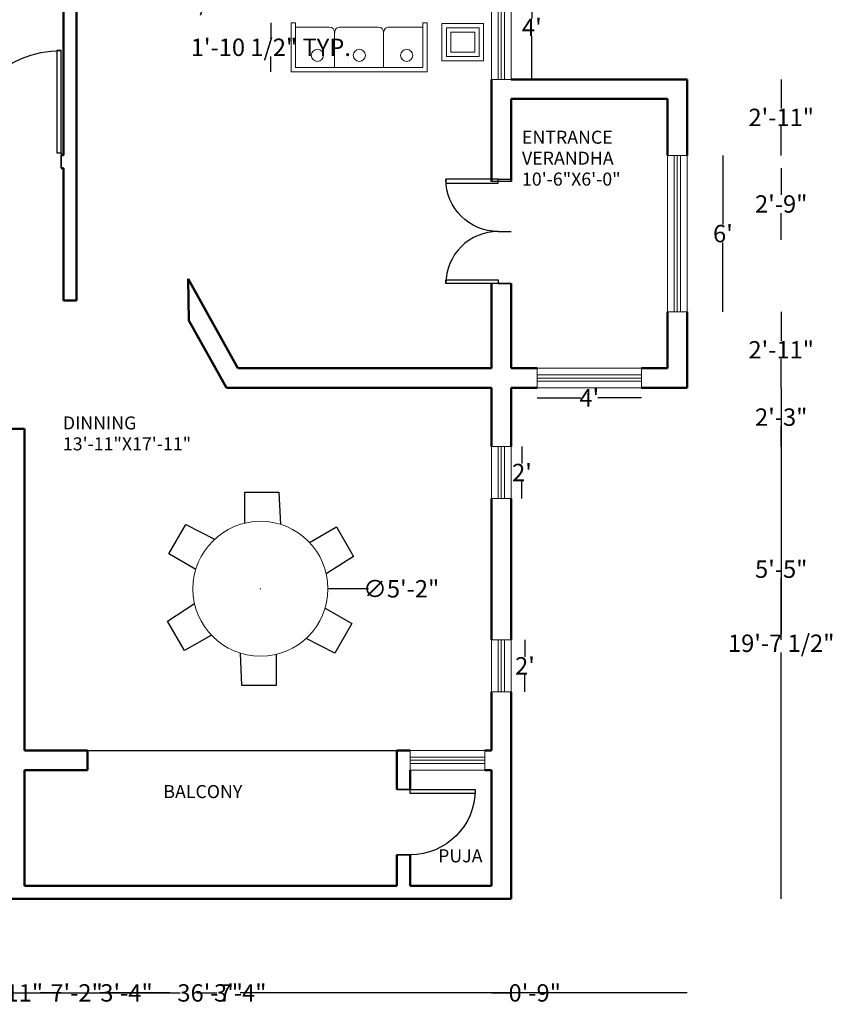
# Model space of a CAD drawing. Units: inches. Extents: x -135167 to -134597, y 156853 to 157819.
# Tile 2 of 5: x -134971 to -134597, y 156853 to 157306. Entities that reach past the tile are written whole.
import ezdxf

# ---------------------------------------------------------------- set-up
doc = ezdxf.new("R2010")
doc.units = ezdxf.units.IN
doc.header["$MEASUREMENT"] = 0
for name, color, linetype, lineweight in [('A-ANNO-DIMS', 4, 'Continuous', 18), ('A-AREA-IDEN', 76, 'Continuous', 25), ('A-FURN', 1, 'Continuous', 18), ('doors', 5, 'Continuous', 25), ('walls', 2, 'Continuous', 50), ('window', 6, 'Continuous', 18)]:
    doc.layers.add(name, color=color, linetype=linetype, lineweight=lineweight)
doc.layers.add('funiture', color=1, linetype='Continuous')
doc.styles.get("Standard").update_dxf_attribs({"font": 'arial.ttf'})
doc.dimstyles.get("Standard").update_dxf_attribs({"dimtxt": 8, "dimasz": 0.18, "dimexe": 0.18, "dimexo": 0.0625, "dimgap": 0.09, "dimtad": 0, "dimtih": 1, "dimtoh": 1, "dimdec": 0, "dimzin": 0, "dimdsep": 46, "dimlunit": 3, "dimtxsty": 'Standard', "dimblk": 'ARCHTICK', "dimcen": 0.09, "dimse1": 1, "dimse2": 1, "dimadec": 0, "dimazin": 0, "dimtfac": 1, "dimtdec": 0, "dimtofl": 0, "dimtmove": 0, "dimatfit": 3, "dimldrblk": 'DOTSMALL', "dimfxl": 1, "dimtolj": 1, "dimtzin": 0, "dimarcsym": 0})

# ---------------------------------------------------------------- blocks, each defined once
blk = doc.blocks.new('*U10')
for p, q in [((0, 0), (0, -6)), ((24, 0), (24, -6))]:
    blk.add_line(p, q)
blk.add_lwpolyline([(0, 0), (0, 24), (1.75, 24), (1.75, 0)], close=True)
blk.add_arc((0, 0), 24, 360, 90)
blk = doc.blocks.new('*U6')
for p, q in [((0, 0), (0, -6)), ((40, 0), (40, -6))]:
    blk.add_line(p, q)
blk.add_lwpolyline([(0, 0), (0, 40), (1.75, 40), (1.75, 0)], close=True)
blk.add_arc((0, 0), 40, 0, 90)
blk = doc.blocks.new('*U7')
for p, q in [((0, 0), (0, 6)), ((30, 0), (30, 6))]:
    blk.add_line(p, q)
blk.add_lwpolyline([(0, 0), (0, -30), (1.75, -30), (1.75, 0)], close=True)
blk.add_arc((0, 0), 30, 270, 0)
blk = doc.blocks.new('*U17')
at = {"layer": 'funiture'}
for p, q in [((-8.21, -6.85), (-8.21, 7.41)), ((-8.21, 7.41), (7.48, 7.41)), ((7.48, 7.41), (8.21, -7.41))]:
    blk.add_line(p, q, dxfattribs=at)
blk = doc.blocks.new('*U18')
at = {"layer": 'A-FURN', "transparency": 16777216}
blk.add_blockref('*U17', (-134859.22, 157081.35), dxfattribs=at)
for p, rotation in [((-134891.84, 157063.7), 59.99999999999999), ((-134827.62, 157061.93), 300), ((-134892.87, 157026.62), 119.9999999999999), ((-134828.64, 157024.85), 239.9999999999999), ((-134861.27, 157007.2), 180)]:
    blk.add_blockref('*U17', p, dxfattribs=dict(at, rotation=rotation))
blk = doc.blocks.new('_ArchTick')
at = {"color": 0, "linetype": 'ByBlock', "const_width": 0.15}
blk.add_lwpolyline([(-0.5, -0.5), (0.5, 0.5)], dxfattribs=at)
blk = doc.blocks.new('*D21')
at = {"layer": 'A-ANNO-DIMS', "color": 0, "lineweight": -2, "transparency": 16777216}
for p, q in [((-134738.49, 157020.8), (-134738.49, 157012.91)), ((-134738.49, 156996.8), (-134738.49, 157004.69))]:
    blk.add_line(p, q, dxfattribs=at)
at = {"layer": 'Defpoints', "color": 0, "transparency": 16777216}
for p in [(-134744.89, 157020.8), (-134738.49, 157020.8), (-134744.89, 156996.8)]:
    blk.add_point(p, dxfattribs=at)
at = {"layer": 'A-ANNO-DIMS', "color": 0, "lineweight": -2, "transparency": 16777216, "xscale": 0.18, "yscale": 0.18, "zscale": 0.18}
for p, rotation in [((-134738.49, 157020.8), 90), ((-134738.49, 156996.8), 270)]:
    blk.add_blockref('_ArchTick', p, dxfattribs=dict(at, rotation=rotation))
at = {"layer": 'A-ANNO-DIMS', "color": 0, "transparency": 16777216, "insert": (-134738.49, 157008.8), "char_height": 8, "attachment_point": 5}
blk.add_mtext("\\A1;2'", dxfattribs=at)
blk = doc.blocks.new('_DotSmall')
at = {"color": 0, "linetype": 'ByBlock', "const_width": 0.5}
blk.add_lwpolyline([(-0.0625, 0, 1), (0.0625, 0, 1)], format="xyb", close=True, dxfattribs=at)
blk = doc.blocks.new('*D22')
at = {"layer": 'A-ANNO-DIMS', "color": 0, "lineweight": -2, "transparency": 16777216}
for p, q in [((-134739.87, 157109.8), (-134739.87, 157101.91)), ((-134739.87, 157085.8), (-134739.87, 157093.69))]:
    blk.add_line(p, q, dxfattribs=at)
at = {"layer": 'Defpoints', "color": 0, "transparency": 16777216}
for p in [(-134744.89, 157109.8), (-134739.87, 157109.8), (-134744.89, 157085.8)]:
    blk.add_point(p, dxfattribs=at)
at = {"layer": 'A-ANNO-DIMS', "color": 0, "lineweight": -2, "transparency": 16777216, "xscale": 0.18, "yscale": 0.18, "zscale": 0.18}
for p, rotation in [((-134739.87, 157109.8), 90), ((-134739.87, 157085.8), 270)]:
    blk.add_blockref('_ArchTick', p, dxfattribs=dict(at, rotation=rotation))
at = {"layer": 'A-ANNO-DIMS', "color": 0, "transparency": 16777216, "insert": (-134739.87, 157097.8), "char_height": 8, "attachment_point": 5}
blk.add_mtext("\\A1;2'", dxfattribs=at)
blk = doc.blocks.new('*D23')
at = {"layer": 'A-ANNO-DIMS', "color": 0, "lineweight": -2, "transparency": 16777216}
for p, q in [((-134732.89, 157132.19), (-134712.82, 157132.19)), ((-134684.89, 157132.19), (-134704.95, 157132.19))]:
    blk.add_line(p, q, dxfattribs=at)
at = {"layer": 'Defpoints', "color": 0, "transparency": 16777216}
for p in [(-134732.89, 157136.8), (-134684.89, 157136.8), (-134684.89, 157132.19)]:
    blk.add_point(p, dxfattribs=at)
at = {"layer": 'A-ANNO-DIMS', "color": 0, "lineweight": -2, "transparency": 16777216, "xscale": 0.18, "yscale": 0.18, "zscale": 0.18, "rotation": 180}
blk.add_blockref('_ArchTick', (-134732.89, 157132.19), dxfattribs=at)
at = {"layer": 'A-ANNO-DIMS', "color": 0, "lineweight": -2, "transparency": 16777216, "xscale": 0.18, "yscale": 0.18, "zscale": 0.18}
blk.add_blockref('_ArchTick', (-134684.89, 157132.19), dxfattribs=at)
at = {"layer": 'A-ANNO-DIMS', "color": 0, "transparency": 16777216, "insert": (-134708.89, 157132.19), "char_height": 8, "attachment_point": 5}
blk.add_mtext("\\A1;4'", dxfattribs=at)
blk = doc.blocks.new('*D24')
at = {"layer": 'A-ANNO-DIMS', "color": 0, "lineweight": -2, "transparency": 16777216}
for p, q in [((-134647.38, 157243.8), (-134647.38, 157211.98)), ((-134647.38, 157171.8), (-134647.38, 157203.63))]:
    blk.add_line(p, q, dxfattribs=at)
at = {"layer": 'Defpoints', "color": 0, "transparency": 16777216}
for p in [(-134663.89, 157243.8), (-134647.38, 157243.8), (-134663.89, 157171.8)]:
    blk.add_point(p, dxfattribs=at)
at = {"layer": 'A-ANNO-DIMS', "color": 0, "lineweight": -2, "transparency": 16777216, "xscale": 0.18, "yscale": 0.18, "zscale": 0.18}
for p, rotation in [((-134647.38, 157243.8), 90), ((-134647.38, 157171.8), 270)]:
    blk.add_blockref('_ArchTick', p, dxfattribs=dict(at, rotation=rotation))
at = {"layer": 'A-ANNO-DIMS', "color": 0, "transparency": 16777216, "insert": (-134647.38, 157207.8), "char_height": 8, "attachment_point": 5}
blk.add_mtext("\\A1;6'", dxfattribs=at)
blk = doc.blocks.new('*D25')
at = {"layer": 'A-ANNO-DIMS', "color": 0, "lineweight": -2, "transparency": 16777216}
for p, q in [((-134735.32, 157326.8), (-134735.32, 157306.89)), ((-134735.32, 157278.8), (-134735.32, 157298.71))]:
    blk.add_line(p, q, dxfattribs=at)
at = {"layer": 'Defpoints', "color": 0, "transparency": 16777216}
for p in [(-134747.89, 157326.8), (-134735.32, 157326.8), (-134744.89, 157278.8)]:
    blk.add_point(p, dxfattribs=at)
at = {"layer": 'A-ANNO-DIMS', "color": 0, "lineweight": -2, "transparency": 16777216, "xscale": 0.18, "yscale": 0.18, "zscale": 0.18}
for p, rotation in [((-134735.32, 157326.8), 90), ((-134735.32, 157278.8), 270)]:
    blk.add_blockref('_ArchTick', p, dxfattribs=dict(at, rotation=rotation))
at = {"layer": 'A-ANNO-DIMS', "color": 0, "transparency": 16777216, "insert": (-134735.32, 157302.8), "char_height": 8, "attachment_point": 5}
blk.add_mtext("\\A1;4'", dxfattribs=at)
blk = doc.blocks.new('SOFA-THREE-SEAT')
for p, q in [((20, 4.47), (20, 20.64)), ((42.55, 4.47), (42.55, 20.64)), ((2, 2), (2, 0)), ((60.55, 2), (60.55, 0))]:
    blk.add_line(p, q)
for points in [[(2, 0), (0, 0), (0, 22.64), (62.55, 22.64), (62.55, 0), (60.55, 0)], [(17.53, 2), (2, 2), (2, 20.64), (60.55, 20.64), (60.55, 2), (45.02, 2)], [(40.07, 2), (22.47, 2)]]:
    blk.add_lwpolyline(points)
for centre in [(9.42, 15.02), (31.21, 15.02), (50.51, 15.02)]:
    blk.add_circle(centre, 2.8)
for centre, start, end in [((17.53, 4.47), 270, 0), ((22.47, 4.47), 180, 270), ((40.07, 4.47), 270, 0), ((45.02, 4.47), 180, 270)]:
    blk.add_arc(centre, 2.47, start, end)
blk = doc.blocks.new('TABLE-END')
for points in [[(0, 17.25), (19.14, 17.25), (19.14, 0), (0, 0)], [(2, 15.25), (17.14, 15.25), (17.14, 2), (2, 2)], [(4, 13.25), (15.14, 13.25), (15.14, 4), (4, 4)]]:
    blk.add_lwpolyline(points, close=True)
blk = doc.blocks.new('WIN-24IN')
for p, q in [((0, 24), (9, 24)), ((0, 24), (0, 0)), ((3, 24), (3, 0)), ((4.5, 24), (4.5, 0)), ((6, 24), (6, 0)), ((9, 24), (9, 0)), ((0, 0), (9, 0))]:
    blk.add_line(p, q)
blk = doc.blocks.new('WIN-48IN')
for p, q in [((0, 48), (9, 48)), ((0, 0), (0, 48)), ((3, 0), (3, 48)), ((4.5, 0), (4.5, 48)), ((6, 0), (6, 48)), ((9, 0), (9, 48)), ((0, 0), (9, 0))]:
    blk.add_line(p, q)
blk = doc.blocks.new('*D46')
at = {"layer": 'A-ANNO-DIMS', "color": 0, "lineweight": -2, "transparency": 16777216}
for p, q in [((-134846.08, 157314.27), (-134846.26, 157314.27)), ((-134783.53, 157314.27), (-134846.08, 157314.27))]:
    blk.add_line(p, q, dxfattribs=at)
at = {"layer": 'Defpoints', "color": 0, "transparency": 16777216}
for p in [(-134846.08, 157314.27), (-134846.08, 157304.89), (-134783.53, 157304.89)]:
    blk.add_point(p, dxfattribs=at)
at = {"layer": 'A-ANNO-DIMS', "color": 0, "lineweight": -2, "transparency": 16777216, "xscale": 0.18, "yscale": 0.18, "zscale": 0.18, "rotation": 180}
blk.add_blockref('_ArchTick', (-134846.08, 157314.27), dxfattribs=at)
at = {"layer": 'A-ANNO-DIMS', "color": 0, "lineweight": -2, "transparency": 16777216, "xscale": 0.18, "yscale": 0.18, "zscale": 0.18}
blk.add_blockref('_ArchTick', (-134783.53, 157314.27), dxfattribs=at)
at = {"layer": 'A-ANNO-DIMS', "color": 0, "transparency": 16777216, "insert": (-134896.8, 157314.27), "char_height": 8, "attachment_point": 5}
blk.add_mtext('\\A1;SOFA 5\'-2 1/2" TYP.', dxfattribs=at)
blk = doc.blocks.new('*D47')
at = {"layer": 'A-ANNO-DIMS', "color": 0, "lineweight": -2, "transparency": 16777216}
for p, q in [((-134855.46, 157304.89), (-134855.46, 157297.8)), ((-134855.46, 157282.25), (-134855.46, 157289.34))]:
    blk.add_line(p, q, dxfattribs=at)
at = {"layer": 'Defpoints', "color": 0, "transparency": 16777216}
for p in [(-134846.08, 157304.89), (-134855.46, 157282.25), (-134846.08, 157282.25)]:
    blk.add_point(p, dxfattribs=at)
at = {"layer": 'A-ANNO-DIMS', "color": 0, "lineweight": -2, "transparency": 16777216, "xscale": 0.18, "yscale": 0.18, "zscale": 0.18}
for p, rotation in [((-134855.46, 157304.89), 90), ((-134855.46, 157282.25), 270)]:
    blk.add_blockref('_ArchTick', p, dxfattribs=dict(at, rotation=rotation))
at = {"layer": 'A-ANNO-DIMS', "color": 0, "transparency": 16777216, "insert": (-134855.46, 157293.57), "char_height": 8, "attachment_point": 5}
blk.add_mtext('\\A1;1\'-10 1/2" TYP.', dxfattribs=at)
blk = doc.blocks.new('*D54')
at = {"layer": 'A-ANNO-DIMS', "color": 0, "lineweight": -2, "transparency": 16777216}
for p, q in [((-135102.89, 156858.2), (-134897.21, 156858.2)), ((-134663.89, 156858.2), (-134869.56, 156858.2))]:
    blk.add_line(p, q, dxfattribs=at)
at = {"layer": 'Defpoints', "color": 0, "transparency": 16777216}
for p in [(-134663.89, 157136.8), (-135102.89, 156901.55), (-134663.89, 156858.2)]:
    blk.add_point(p, dxfattribs=at)
at = {"layer": 'A-ANNO-DIMS', "color": 0, "lineweight": -2, "transparency": 16777216, "xscale": 0.18, "yscale": 0.18, "zscale": 0.18, "rotation": 180}
blk.add_blockref('_ArchTick', (-135102.89, 156858.2), dxfattribs=at)
at = {"layer": 'A-ANNO-DIMS', "color": 0, "lineweight": -2, "transparency": 16777216, "xscale": 0.18, "yscale": 0.18, "zscale": 0.18}
blk.add_blockref('_ArchTick', (-134663.89, 156858.2), dxfattribs=at)
at = {"layer": 'A-ANNO-DIMS', "color": 0, "transparency": 16777216, "insert": (-134883.39, 156858.2), "char_height": 8, "attachment_point": 5}
blk.add_mtext('\\A1;36\'-7"', dxfattribs=at)
blk = doc.blocks.new('*D55')
at = {"layer": 'A-ANNO-DIMS', "color": 0, "lineweight": -2, "transparency": 16777216}
for p, q in [((-134620.54, 157136.8), (-134620.54, 157023.4)), ((-134620.54, 156901.55), (-134620.54, 157014.95))]:
    blk.add_line(p, q, dxfattribs=at)
at = {"layer": 'Defpoints', "color": 0, "transparency": 16777216}
for p in [(-134663.89, 157136.8), (-134620.54, 157136.8), (-134744.89, 156901.55)]:
    blk.add_point(p, dxfattribs=at)
at = {"layer": 'A-ANNO-DIMS', "color": 0, "lineweight": -2, "transparency": 16777216, "xscale": 0.18, "yscale": 0.18, "zscale": 0.18}
for p, rotation in [((-134620.54, 157136.8), 90), ((-134620.54, 156901.55), 270)]:
    blk.add_blockref('_ArchTick', p, dxfattribs=dict(at, rotation=rotation))
at = {"layer": 'A-ANNO-DIMS', "color": 0, "transparency": 16777216, "insert": (-134620.54, 157019.18), "char_height": 8, "attachment_point": 5}
blk.add_mtext('\\A1;19\'-7 1/2"', dxfattribs=at)
blk = doc.blocks.new('*D65')
at = {"layer": 'A-ANNO-DIMS', "color": 0, "lineweight": -2, "transparency": 16777216}
for p, q in [((-134620.54, 157278.8), (-134620.54, 157265.41)), ((-134620.54, 157243.8), (-134620.54, 157257.19))]:
    blk.add_line(p, q, dxfattribs=at)
at = {"layer": 'Defpoints', "color": 0, "transparency": 16777216}
for p in [(-134663.89, 157278.8), (-134663.89, 157243.8), (-134620.54, 157243.8)]:
    blk.add_point(p, dxfattribs=at)
at = {"layer": 'A-ANNO-DIMS', "color": 0, "lineweight": -2, "transparency": 16777216, "xscale": 0.18, "yscale": 0.18, "zscale": 0.18}
for p, rotation in [((-134620.54, 157278.8), 90), ((-134620.54, 157243.8), 270)]:
    blk.add_blockref('_ArchTick', p, dxfattribs=dict(at, rotation=rotation))
at = {"layer": 'A-ANNO-DIMS', "color": 0, "transparency": 16777216, "insert": (-134620.54, 157261.3), "char_height": 8, "attachment_point": 5}
blk.add_mtext('\\A1;2\'-11"', dxfattribs=at)
blk = doc.blocks.new('*D66')
at = {"layer": 'A-ANNO-DIMS', "color": 0, "lineweight": -2, "transparency": 16777216}
for p, q in [((-134620.54, 157171.8), (-134620.54, 157158.41)), ((-134620.54, 157136.8), (-134620.54, 157150.19))]:
    blk.add_line(p, q, dxfattribs=at)
at = {"layer": 'Defpoints', "color": 0, "transparency": 16777216}
for p in [(-134663.89, 157171.8), (-134663.89, 157136.8), (-134620.54, 157136.8)]:
    blk.add_point(p, dxfattribs=at)
at = {"layer": 'A-ANNO-DIMS', "color": 0, "lineweight": -2, "transparency": 16777216, "xscale": 0.18, "yscale": 0.18, "zscale": 0.18}
for p, rotation in [((-134620.54, 157171.8), 90), ((-134620.54, 157136.8), 270)]:
    blk.add_blockref('_ArchTick', p, dxfattribs=dict(at, rotation=rotation))
at = {"layer": 'A-ANNO-DIMS', "color": 0, "transparency": 16777216, "insert": (-134620.54, 157154.3), "char_height": 8, "attachment_point": 5}
blk.add_mtext('\\A1;2\'-11"', dxfattribs=at)
blk = doc.blocks.new('*D67')
at = {"layer": 'A-ANNO-DIMS', "color": 0, "lineweight": -2, "transparency": 16777216}
for p, q in [((-134744.89, 157806.8), (-134732.89, 157806.8)), ((-134732.89, 157806.8), (-134732.71, 157806.8))]:
    blk.add_line(p, q, dxfattribs=at)
at = {"layer": 'Defpoints', "color": 0, "transparency": 16777216}
for p in [(-134732.89, 157806.8), (-134744.89, 157145.8), (-134732.89, 157145.8)]:
    blk.add_point(p, dxfattribs=at)
at = {"layer": 'A-ANNO-DIMS', "color": 0, "lineweight": -2, "transparency": 16777216, "xscale": 0.18, "yscale": 0.18, "zscale": 0.18, "rotation": 180}
blk.add_blockref('_ArchTick', (-134744.89, 157806.8), dxfattribs=at)
at = {"layer": 'A-ANNO-DIMS', "color": 0, "lineweight": -2, "transparency": 16777216, "xscale": 0.18, "yscale": 0.18, "zscale": 0.18}
blk.add_blockref('_ArchTick', (-134732.89, 157806.8), dxfattribs=at)
at = {"layer": 'A-ANNO-DIMS', "color": 0, "transparency": 16777216, "insert": (-134722.36, 157806.8), "char_height": 8, "attachment_point": 5}
blk.add_mtext('\\A1;1\'-0"', dxfattribs=at)
blk = doc.blocks.new('*D68')
at = {"layer": 'A-ANNO-DIMS', "color": 0, "lineweight": -2, "transparency": 16777216}
for p, q in [((-134620.54, 157136.8), (-134620.54, 157127.48)), ((-134620.54, 157109.8), (-134620.54, 157119.12))]:
    blk.add_line(p, q, dxfattribs=at)
at = {"layer": 'Defpoints', "color": 0, "transparency": 16777216}
for p in [(-134744.89, 157136.8), (-134744.89, 157109.8), (-134620.54, 157109.8)]:
    blk.add_point(p, dxfattribs=at)
at = {"layer": 'A-ANNO-DIMS', "color": 0, "lineweight": -2, "transparency": 16777216, "xscale": 0.18, "yscale": 0.18, "zscale": 0.18}
for p, rotation in [((-134620.54, 157136.8), 90), ((-134620.54, 157109.8), 270)]:
    blk.add_blockref('_ArchTick', p, dxfattribs=dict(at, rotation=rotation))
at = {"layer": 'A-ANNO-DIMS', "color": 0, "transparency": 16777216, "insert": (-134620.54, 157123.3), "char_height": 8, "attachment_point": 5}
blk.add_mtext('\\A1;2\'-3"', dxfattribs=at)
blk = doc.blocks.new('*D69')
at = {"layer": 'A-ANNO-DIMS', "color": 0, "lineweight": -2, "transparency": 16777216}
for p, q in [((-134620.54, 157085.8), (-134620.54, 157057.46)), ((-134620.54, 157020.8), (-134620.54, 157049.14))]:
    blk.add_line(p, q, dxfattribs=at)
at = {"layer": 'Defpoints', "color": 0, "transparency": 16777216}
for p in [(-134744.89, 157085.8), (-134744.89, 157020.8), (-134620.54, 157020.8)]:
    blk.add_point(p, dxfattribs=at)
at = {"layer": 'A-ANNO-DIMS', "color": 0, "lineweight": -2, "transparency": 16777216, "xscale": 0.18, "yscale": 0.18, "zscale": 0.18}
for p, rotation in [((-134620.54, 157085.8), 90), ((-134620.54, 157020.8), 270)]:
    blk.add_blockref('_ArchTick', p, dxfattribs=dict(at, rotation=rotation))
at = {"layer": 'A-ANNO-DIMS', "color": 0, "transparency": 16777216, "insert": (-134620.54, 157053.3), "char_height": 8, "attachment_point": 5}
blk.add_mtext('\\A1;5\'-5"', dxfattribs=at)
blk = doc.blocks.new('*D72')
at = {"layer": 'A-ANNO-DIMS', "color": 0, "lineweight": -2, "transparency": 16777216}
for p, q in [((-134753.885731, 156858.200753), (-134744.885731, 156858.200753)), ((-134744.885731, 156858.200753), (-134744.705731, 156858.200753))]:
    blk.add_line(p, q, dxfattribs=at)
at = {"layer": 'Defpoints', "color": 0, "transparency": 16777216}
for p in [(-134753.885731, 157278.800753), (-134744.885731, 157278.800753), (-134744.885731, 156858.200753)]:
    blk.add_point(p, dxfattribs=at)
at = {"layer": 'A-ANNO-DIMS', "color": 0, "lineweight": -2, "transparency": 16777216, "xscale": 0.18, "yscale": 0.18, "zscale": 0.18, "rotation": 180}
blk.add_blockref('_ArchTick', (-134753.885731, 156858.200753), dxfattribs=at)
at = {"layer": 'A-ANNO-DIMS', "color": 0, "lineweight": -2, "transparency": 16777216, "xscale": 0.18, "yscale": 0.18, "zscale": 0.18}
blk.add_blockref('_ArchTick', (-134744.885731, 156858.200753), dxfattribs=at)
at = {"layer": 'A-ANNO-DIMS', "color": 0, "transparency": 16777216, "insert": (-134733.982716, 156858.200753), "char_height": 8, "attachment_point": 5}
blk.add_mtext('\\A1;0\'-9"', dxfattribs=at)
blk = doc.blocks.new('*D79')
at = {"layer": 'A-ANNO-DIMS', "color": 0, "lineweight": -2, "transparency": 16777216}
for p, q in [((-135146.24, 157231.8), (-135146.24, 157212.48)), ((-135146.24, 157184.8), (-135146.24, 157204.12))]:
    blk.add_line(p, q, dxfattribs=at)
at = {"layer": 'Defpoints', "color": 0, "transparency": 16777216}
for p in [(-135146.24, 157231.8), (-134753.89, 157231.8), (-134753.89, 157184.8)]:
    blk.add_point(p, dxfattribs=at)
at = {"layer": 'A-ANNO-DIMS', "color": 0, "lineweight": -2, "transparency": 16777216, "xscale": 0.18, "yscale": 0.18, "zscale": 0.18}
for p, rotation in [((-135146.24, 157231.8), 90), ((-135146.24, 157184.8), 270)]:
    blk.add_blockref('_ArchTick', p, dxfattribs=dict(at, rotation=rotation))
at = {"layer": 'A-ANNO-DIMS', "color": 0, "transparency": 16777216, "insert": (-135146.24, 157208.3), "char_height": 8, "attachment_point": 5}
blk.add_mtext('\\A1;3\'-11"', dxfattribs=at)
blk = doc.blocks.new('*D80')
at = {"layer": 'A-ANNO-DIMS', "color": 0, "lineweight": -2, "transparency": 16777216}
for p, q in [((-135146.24, 157184.8), (-135146.24, 157169.48)), ((-135146.24, 157145.8), (-135146.24, 157161.12))]:
    blk.add_line(p, q, dxfattribs=at)
at = {"layer": 'Defpoints', "color": 0, "transparency": 16777216}
for p in [(-135146.24, 157184.8), (-134753.89, 157184.8), (-134753.89, 157145.8)]:
    blk.add_point(p, dxfattribs=at)
at = {"layer": 'A-ANNO-DIMS', "color": 0, "lineweight": -2, "transparency": 16777216, "xscale": 0.18, "yscale": 0.18, "zscale": 0.18}
for p, rotation in [((-135146.24, 157184.8), 90), ((-135146.24, 157145.8), 270)]:
    blk.add_blockref('_ArchTick', p, dxfattribs=dict(at, rotation=rotation))
at = {"layer": 'A-ANNO-DIMS', "color": 0, "transparency": 16777216, "insert": (-135146.24, 157165.3), "char_height": 8, "attachment_point": 5}
blk.add_mtext('\\A1;3\'-3"', dxfattribs=at)
blk = doc.blocks.new('*D81')
at = {"layer": 'A-ANNO-DIMS', "color": 0, "lineweight": -2, "transparency": 16777216}
for p, q in [((-134941.89, 156858.2), (-134932.61, 156858.2)), ((-134901.89, 156858.2), (-134911.17, 156858.2))]:
    blk.add_line(p, q, dxfattribs=at)
at = {"layer": 'Defpoints', "color": 0, "transparency": 16777216}
for p in [(-134941.89, 157473.94), (-134901.89, 157473.94), (-134901.89, 156858.2)]:
    blk.add_point(p, dxfattribs=at)
at = {"layer": 'A-ANNO-DIMS', "color": 0, "lineweight": -2, "transparency": 16777216, "xscale": 0.18, "yscale": 0.18, "zscale": 0.18, "rotation": 180}
blk.add_blockref('_ArchTick', (-134941.89, 156858.2), dxfattribs=at)
at = {"layer": 'A-ANNO-DIMS', "color": 0, "lineweight": -2, "transparency": 16777216, "xscale": 0.18, "yscale": 0.18, "zscale": 0.18}
blk.add_blockref('_ArchTick', (-134901.89, 156858.2), dxfattribs=at)
at = {"layer": 'A-ANNO-DIMS', "color": 0, "transparency": 16777216, "insert": (-134921.89, 156858.2), "char_height": 8, "attachment_point": 5}
blk.add_mtext('\\A1;3\'-4"', dxfattribs=at)
blk = doc.blocks.new('*D82')
at = {"layer": 'A-ANNO-DIMS', "color": 0, "lineweight": -2, "transparency": 16777216}
for p, q in [((-134889.54, 156858.2), (-134880.26, 156858.2)), ((-134849.54, 156858.2), (-134858.82, 156858.2))]:
    blk.add_line(p, q, dxfattribs=at)
at = {"layer": 'Defpoints', "color": 0, "transparency": 16777216}
for p in [(-134889.54, 157473.94), (-134849.54, 157473.94), (-134849.54, 156858.2)]:
    blk.add_point(p, dxfattribs=at)
at = {"layer": 'A-ANNO-DIMS', "color": 0, "lineweight": -2, "transparency": 16777216, "xscale": 0.18, "yscale": 0.18, "zscale": 0.18, "rotation": 180}
blk.add_blockref('_ArchTick', (-134889.54, 156858.2), dxfattribs=at)
at = {"layer": 'A-ANNO-DIMS', "color": 0, "lineweight": -2, "transparency": 16777216, "xscale": 0.18, "yscale": 0.18, "zscale": 0.18}
blk.add_blockref('_ArchTick', (-134849.54, 156858.2), dxfattribs=at)
at = {"layer": 'A-ANNO-DIMS', "color": 0, "transparency": 16777216, "insert": (-134869.54, 156858.2), "char_height": 8, "attachment_point": 5}
blk.add_mtext('\\A1;3\'-4"', dxfattribs=at)
blk = doc.blocks.new('*D84')
at = {"layer": 'A-ANNO-DIMS', "color": 0, "lineweight": -2, "transparency": 16777216}
for p, q in [((-134998.89, 156858.2), (-134989.21, 156858.2)), ((-134951.89, 156858.2), (-134961.56, 156858.2))]:
    blk.add_line(p, q, dxfattribs=at)
at = {"layer": 'Defpoints', "color": 0, "transparency": 16777216}
for p in [(-134998.89, 157237.94), (-134951.89, 157237.94), (-134951.89, 156858.2)]:
    blk.add_point(p, dxfattribs=at)
at = {"layer": 'A-ANNO-DIMS', "color": 0, "lineweight": -2, "transparency": 16777216, "xscale": 0.18, "yscale": 0.18, "zscale": 0.18, "rotation": 180}
blk.add_blockref('_ArchTick', (-134998.89, 156858.2), dxfattribs=at)
at = {"layer": 'A-ANNO-DIMS', "color": 0, "lineweight": -2, "transparency": 16777216, "xscale": 0.18, "yscale": 0.18, "zscale": 0.18}
blk.add_blockref('_ArchTick', (-134951.89, 156858.2), dxfattribs=at)
at = {"layer": 'A-ANNO-DIMS', "color": 0, "transparency": 16777216, "insert": (-134975.39, 156858.2), "char_height": 8, "attachment_point": 5}
blk.add_mtext('\\A1;3\'-11"', dxfattribs=at)
blk = doc.blocks.new('*D85')
at = {"layer": 'A-ANNO-DIMS', "color": 0, "lineweight": -2, "transparency": 16777216}
for p, q in [((-134620.54, 157237.94), (-134620.54, 157225.62)), ((-134620.54, 157204.94), (-134620.54, 157217.27))]:
    blk.add_line(p, q, dxfattribs=at)
at = {"layer": 'Defpoints', "color": 0, "transparency": 16777216}
for p in [(-135004.89, 157237.94), (-135004.89, 157204.94), (-134620.54, 157204.94)]:
    blk.add_point(p, dxfattribs=at)
at = {"layer": 'A-ANNO-DIMS', "color": 0, "lineweight": -2, "transparency": 16777216, "xscale": 0.18, "yscale": 0.18, "zscale": 0.18}
for p, rotation in [((-134620.54, 157237.94), 90), ((-134620.54, 157204.94), 270)]:
    blk.add_blockref('_ArchTick', p, dxfattribs=dict(at, rotation=rotation))
at = {"layer": 'A-ANNO-DIMS', "color": 0, "transparency": 16777216, "insert": (-134620.54, 157221.44), "char_height": 8, "attachment_point": 5}
blk.add_mtext('\\A1;2\'-9"', dxfattribs=at)
blk = doc.blocks.new('*D90')
at = {"layer": 'A-ANNO-DIMS', "color": 0, "lineweight": -2, "transparency": 16777216}
for p, q in [((-134791.39, 157806.8), (-134756.89, 157806.8)), ((-134756.89, 157806.8), (-134756.71, 157806.8))]:
    blk.add_line(p, q, dxfattribs=at)
at = {"layer": 'Defpoints', "color": 0, "transparency": 16777216}
for p in [(-134756.89, 157806.8), (-134791.39, 156969.8), (-134756.89, 156969.8)]:
    blk.add_point(p, dxfattribs=at)
at = {"layer": 'A-ANNO-DIMS', "color": 0, "lineweight": -2, "transparency": 16777216, "xscale": 0.18, "yscale": 0.18, "zscale": 0.18, "rotation": 180}
blk.add_blockref('_ArchTick', (-134791.39, 157806.8), dxfattribs=at)
at = {"layer": 'A-ANNO-DIMS', "color": 0, "lineweight": -2, "transparency": 16777216, "xscale": 0.18, "yscale": 0.18, "zscale": 0.18}
blk.add_blockref('_ArchTick', (-134756.89, 157806.8), dxfattribs=at)
at = {"layer": 'A-ANNO-DIMS', "color": 0, "transparency": 16777216, "insert": (-134733.49, 157806.8), "char_height": 8, "attachment_point": 5}
blk.add_mtext('\\A1;2\'-10 1/2"', dxfattribs=at)
blk = doc.blocks.new('*D91')
at = {"layer": 'A-ANNO-DIMS', "color": 0, "lineweight": -2, "transparency": 16777216}
for p, q in [((-135146.24, 156951.78), (-135146.24, 156940.95)), ((-135146.24, 156921.78), (-135146.24, 156932.6))]:
    blk.add_line(p, q, dxfattribs=at)
at = {"layer": 'Defpoints', "color": 0, "transparency": 16777216}
for p in [(-134797.39, 156951.78), (-135146.24, 156921.78), (-134797.39, 156921.78)]:
    blk.add_point(p, dxfattribs=at)
at = {"layer": 'A-ANNO-DIMS', "color": 0, "lineweight": -2, "transparency": 16777216, "xscale": 0.18, "yscale": 0.18, "zscale": 0.18}
for p, rotation in [((-135146.24, 156951.78), 90), ((-135146.24, 156921.78), 270)]:
    blk.add_blockref('_ArchTick', p, dxfattribs=dict(at, rotation=rotation))
at = {"layer": 'A-ANNO-DIMS', "color": 0, "transparency": 16777216, "insert": (-135146.24, 156936.78), "char_height": 8, "attachment_point": 5}
blk.add_mtext('\\A1;2\'-6"', dxfattribs=at)
blk = doc.blocks.new('*D92')
at = {"layer": 'A-ANNO-DIMS', "color": 0, "lineweight": -2, "transparency": 16777216}
for p, q in [((-134987.89, 156858.2), (-134955.58, 156858.2)), ((-134901.89, 156858.2), (-134934.2, 156858.2))]:
    blk.add_line(p, q, dxfattribs=at)
at = {"layer": 'Defpoints', "color": 0, "transparency": 16777216}
for p in [(-134987.89, 157647.94), (-134901.89, 157647.94), (-134901.89, 156858.2)]:
    blk.add_point(p, dxfattribs=at)
at = {"layer": 'A-ANNO-DIMS', "color": 0, "lineweight": -2, "transparency": 16777216, "xscale": 0.18, "yscale": 0.18, "zscale": 0.18, "rotation": 180}
blk.add_blockref('_ArchTick', (-134987.89, 156858.2), dxfattribs=at)
at = {"layer": 'A-ANNO-DIMS', "color": 0, "lineweight": -2, "transparency": 16777216, "xscale": 0.18, "yscale": 0.18, "zscale": 0.18}
blk.add_blockref('_ArchTick', (-134901.89, 156858.2), dxfattribs=at)
at = {"layer": 'A-ANNO-DIMS', "color": 0, "transparency": 16777216, "insert": (-134944.89, 156858.2), "char_height": 8, "attachment_point": 5}
blk.add_mtext('\\A1;7\'-2"', dxfattribs=at)
blk = doc.blocks.new('*D98')
at = {"layer": 'A-ANNO-DIMS', "color": 0, "lineweight": -2, "transparency": 16777216}
for p, q in [((-134860.33, 157044.27), (-134860.15, 157044.27)), ((-134860.24, 157044.18), (-134860.24, 157044.36)), ((-134810.53, 157044.27), (-134829.17, 157044.27))]:
    blk.add_line(p, q, dxfattribs=at)
at = {"layer": 'Defpoints', "color": 0, "transparency": 16777216}
for p in [(-134891.32, 157044.27), (-134829.17, 157044.27)]:
    blk.add_point(p, dxfattribs=at)
at = {"layer": 'A-ANNO-DIMS', "color": 0, "lineweight": -2, "transparency": 16777216, "xscale": 0.18, "yscale": 0.18, "zscale": 0.18, "rotation": 179.9992642822033}
blk.add_blockref('_ArchTick', (-134829.17, 157044.27), dxfattribs=at)
at = {"layer": 'A-ANNO-DIMS', "color": 0, "transparency": 16777216, "insert": (-134795.45, 157044.27), "char_height": 8, "attachment_point": 5}
blk.add_mtext('\\A1;∅5\'-2"', dxfattribs=at)

msp = doc.modelspace()

# ---------------------------------------------------------------- linework, layer by layer
at = {"layer": 'A-FURN'}
msp.add_circle((-134860.24, 157044.27), 31.07, dxfattribs=at)
at = {"layer": 'doors'}
for p, q in [((-134951.89, 157237.94), (-134951.89, 157243.94)), ((-134744.89, 157231.8), (-134753.89, 157231.8)), ((-134744.89, 157184.8), (-134753.89, 157184.8)), ((-134939.89, 156969.8), (-134797.39, 156969.8)), ((-134797.39, 156951.78), (-134791.39, 156951.78)), ((-134797.39, 156921.78), (-134791.39, 156921.78))]:
    msp.add_line(p, q, dxfattribs=at)
at = {"layer": 'walls'}
for p, q in [((-134944.89, 157176.94), (-134944.89, 157473.94)), ((-134950.89, 157243.94), (-134950.89, 157395.94)), ((-134753.89, 157231.8), (-134753.89, 157278.8)), ((-134663.89, 157278.8), (-134744.89, 157278.8)), ((-134663.89, 157243.8), (-134663.89, 157278.8)), ((-134672.89, 157269.8), (-134744.89, 157269.8)), ((-134744.89, 157231.8), (-134744.89, 157269.8)), ((-134672.89, 157243.8), (-134672.89, 157269.8)), ((-134951.89, 157243.94), (-134950.89, 157243.94)), ((-134951.89, 157237.94), (-134950.89, 157237.94)), ((-134950.89, 157176.94), (-134950.89, 157237.94)), ((-134893.49, 157186.94), (-134870.64, 157145.8)), ((-134893.18, 157167.85), (-134893.49, 157186.94)), ((-134753.89, 157145.8), (-134753.89, 157184.8)), ((-134744.89, 157145.8), (-134744.89, 157184.8)), ((-134950.89, 157176.94), (-134944.89, 157176.94)), ((-134893.18, 157167.85), (-134875.93, 157136.8)), ((-134672.89, 157145.8), (-134672.89, 157171.8)), ((-134663.89, 157136.8), (-134663.89, 157171.8)), ((-134870.64, 157145.8), (-134753.89, 157145.8)), ((-134744.89, 157145.8), (-134732.89, 157145.8)), ((-134684.89, 157145.8), (-134672.89, 157145.8)), ((-134875.93, 157136.8), (-134753.89, 157136.8)), ((-134753.89, 157109.8), (-134753.89, 157136.8)), ((-134744.89, 157136.8), (-134732.89, 157136.8)), ((-134744.89, 157109.8), (-134744.89, 157136.8)), ((-134684.89, 157136.8), (-134663.89, 157136.8)), ((-134974.89, 157117.94), (-134968.89, 157117.94)), ((-134968.89, 156969.8), (-134968.89, 157117.94)), ((-134753.89, 157020.8), (-134753.89, 157085.8)), ((-134744.89, 157020.8), (-134744.89, 157085.8)), ((-134753.89, 156969.8), (-134753.89, 156996.8)), ((-134744.89, 156901.55), (-134744.89, 156996.8)), ((-134968.89, 156969.8), (-134939.89, 156969.8)), ((-134939.89, 156969.8), (-134939.89, 156960.8)), ((-134797.39, 156951.78), (-134797.39, 156969.8)), ((-134797.39, 156969.8), (-134791.39, 156969.8)), ((-134756.89, 156969.8), (-134753.89, 156969.8)), ((-134968.89, 156907.55), (-134968.89, 156960.8)), ((-134968.89, 156960.8), (-134939.89, 156960.8)), ((-134791.39, 156951.78), (-134791.39, 156960.8)), ((-134756.89, 156960.8), (-134753.89, 156960.8)), ((-134753.89, 156907.55), (-134753.89, 156960.8)), ((-134797.39, 156907.55), (-134797.39, 156921.78)), ((-134791.39, 156907.55), (-134791.39, 156921.78)), ((-134968.89, 156907.55), (-134797.39, 156907.55)), ((-134791.39, 156907.55), (-134753.89, 156907.55)), ((-135102.89, 156901.55), (-134744.89, 156901.55))]:
    msp.add_line(p, q, dxfattribs=at)
at = {"layer": 'window'}
for p, q in [((-134672.89, 157243.8), (-134663.89, 157243.8)), ((-134672.89, 157243.8), (-134672.89, 157171.8)), ((-134669.89, 157243.8), (-134669.89, 157171.8)), ((-134668.39, 157243.8), (-134668.39, 157171.8)), ((-134666.89, 157243.8), (-134666.89, 157171.8)), ((-134663.89, 157243.8), (-134663.89, 157171.8)), ((-134672.89, 157171.8), (-134663.89, 157171.8)), ((-134791.39, 156960.8), (-134791.39, 156969.8)), ((-134756.89, 156969.8), (-134791.39, 156969.8)), ((-134756.89, 156960.8), (-134756.89, 156969.8)), ((-134756.89, 156966.8), (-134791.39, 156966.8)), ((-134756.89, 156965.3), (-134791.39, 156965.3)), ((-134756.89, 156963.8), (-134791.39, 156963.8)), ((-134756.89, 156960.8), (-134791.39, 156960.8))]:
    msp.add_line(p, q, dxfattribs=at)

# ---------------------------------------------------------------- block references
at = {"layer": 'A-FURN', "rotation": 180}
msp.add_blockref('SOFA-THREE-SEAT', (-134783.53, 157304.89), dxfattribs=at)
at = {"layer": 'A-FURN'}
for name, p in [('TABLE-END', (-134776.68, 157287.34)), ('*U18', (0, 0))]:
    msp.add_blockref(name, p, dxfattribs=at)
at = {"layer": 'doors', "xscale": -1.177072109473595, "yscale": 1.177072109473595, "zscale": 1.177072109473595}
msp.add_blockref('*U6', (-134951.89, 157245.01), dxfattribs=at)
at = {"layer": 'doors', "xscale": -1, "rotation": 90}
for name, p in [('*U10', (-134750.89, 157232.8)), ('*U7', (-134791.39, 156951.78))]:
    msp.add_blockref(name, p, dxfattribs=at)
at = {"layer": 'doors', "rotation": 90}
msp.add_blockref('*U10', (-134750.89, 157184.8), dxfattribs=at)
at = {"layer": 'window'}
for p, rotation in [((-134744.89, 157326.8), 180), ((-134732.89, 157145.8), 269.9999999999874)]:
    msp.add_blockref('WIN-48IN', p, dxfattribs=dict(at, rotation=rotation))
for p in [(-134753.89, 157085.8), (-134753.89, 156996.8)]:
    msp.add_blockref('WIN-24IN', p, dxfattribs=at)

# ---------------------------------------------------------------- texts
at = {"layer": 'A-AREA-IDEN'}
for s, p in [('ENTRANCE ', (-134739.86, 157249.17)), ('VERANDHA', (-134739.86, 157239.53)), ('10\'-6"X6\'-0"', (-134739.86, 157229.89)), ('DINNING ', (-134951.18, 157117.62)), ('13\'-11"X17\'-11"', (-134951.18, 157107.99)), ('BALCONY', (-134904.94, 156947.9)), ('PUJA', (-134778.47, 156918.31))]:
    msp.add_text(s, height=6, dxfattribs=at).set_placement(p)

# ---------------------------------------------------------------- dimensions: what is measured, and where the dimension line sits
at = {"layer": 'A-ANNO-DIMS'}
for base, p1, p2, override, picture, middle in [((-134756.89, 157806.8), (-134791.39, 156969.8), (-134756.89, 156969.8), {"dimdec": 1, "dimlfac": 1, "dimrnd": 0, "dimzin": 1, "dimdsep": 46, "dimlunit": 4, "dimfrac": 2}, '*D90', (-134733.49, 157806.8)), ((-134732.89, 157806.8), (-134744.89, 157145.8), (-134732.89, 157145.8), {"dimdec": 1, "dimlfac": 1, "dimrnd": 0, "dimzin": 1, "dimdsep": 46, "dimlunit": 4, "dimfrac": 2}, '*D67', (-134722.36, 157806.8)), ((-134901.89, 156858.2), (-134987.89, 157647.94), (-134901.89, 157647.94), {"dimdec": 1, "dimlfac": 1, "dimrnd": 0, "dimzin": 1, "dimdsep": 46, "dimlunit": 4, "dimfrac": 2}, '*D92', (-134944.89, 156858.2)), ((-134901.89, 156858.2), (-134941.89, 157473.94), (-134901.89, 157473.94), {"dimdec": 1, "dimlfac": 1, "dimrnd": 0, "dimzin": 1, "dimdsep": 46, "dimlunit": 4, "dimfrac": 2}, '*D81', (-134921.89, 156858.2)), ((-134849.54, 156858.2), (-134889.54, 157473.94), (-134849.54, 157473.94), {"dimdec": 1, "dimlfac": 1, "dimrnd": 0, "dimzin": 1, "dimdsep": 46, "dimlunit": 4, "dimfrac": 2}, '*D82', (-134869.54, 156858.2)), ((-134744.89, 156858.2), (-134753.89, 157278.8), (-134744.89, 157278.8), {"dimdec": 1, "dimlfac": 1, "dimrnd": 0, "dimzin": 1, "dimdsep": 46, "dimlunit": 4, "dimfrac": 2}, '*D72', (-134733.98, 156858.2)), ((-134951.89, 156858.2), (-134998.89, 157237.94), (-134951.89, 157237.94), {"dimdec": 1, "dimlfac": 1, "dimrnd": 0, "dimzin": 1, "dimdsep": 46, "dimlunit": 4, "dimfrac": 2}, '*D84', (-134975.39, 156858.2)), ((-134663.89, 156858.2), (-135102.89, 156901.55), (-134663.89, 157136.8), {"dimdec": 1, "dimlfac": 1, "dimrnd": 0, "dimzin": 1, "dimdsep": 46, "dimlunit": 4, "dimfrac": 2}, '*D54', (-134883.39, 156858.2)), ((-134684.89, 157132.19), (-134732.89, 157136.8), (-134684.89, 157136.8), {"dimclrd": 0, "dimclre": 0, "dimclrt": 0}, '*D23', (-134708.89, 157132.19))]:
    dim = msp.add_linear_dim(base=base, p1=p1, p2=p2, dimstyle='Standard', override=override, dxfattribs=at)
    dim.commit()
    dim.dimension.update_dxf_attribs({"geometry": picture, "text_midpoint": middle})
for base, p1, p2, angle, text, picture, middle in [((-134846.0812, 157314.271), (-134783.5338, 157304.8889), (-134846.0812, 157304.8889), 180, 'SOFA <> TYP.', '*D46', (-134896.8014, 157314.271)), ((-134855.46, 157282.25), (-134846.08, 157304.89), (-134846.08, 157282.25), 270, '<> TYP.', '*D47', (-134855.46, 157293.57))]:
    dim = msp.add_linear_dim(base=base, p1=p1, p2=p2, angle=angle, text=text, dimstyle='Standard', override={"dimdec": 1, "dimlfac": 1, "dimrnd": 0, "dimzin": 1, "dimdsep": 46, "dimlunit": 4, "dimfrac": 2}, dxfattribs=at)
    dim.commit()
    dim.dimension.update_dxf_attribs({"geometry": picture, "text_midpoint": middle})
for base, p1, p2, override, picture, middle in [((-134735.32, 157326.8), (-134744.89, 157278.8), (-134747.89, 157326.8), {"dimclrd": 0, "dimclre": 0, "dimclrt": 0}, '*D25', (-134735.32, 157302.8)), ((-134620.54, 157243.8), (-134663.89, 157278.8), (-134663.89, 157243.8), {"dimdec": 1, "dimlfac": 1, "dimrnd": 0, "dimzin": 1, "dimdsep": 46, "dimlunit": 4, "dimfrac": 2}, '*D65', (-134620.54, 157261.3)), ((-134647.38, 157243.8), (-134663.89, 157171.8), (-134663.89, 157243.8), {"dimclrd": 0, "dimclre": 0, "dimclrt": 0}, '*D24', (-134647.38, 157207.8)), ((-134620.54, 157204.94), (-135004.89, 157237.94), (-135004.89, 157204.94), {"dimdec": 1, "dimlfac": 1, "dimrnd": 0, "dimzin": 1, "dimdsep": 46, "dimlunit": 4, "dimfrac": 2}, '*D85', (-134620.54, 157221.44)), ((-135146.24, 157231.8), (-134753.89, 157184.8), (-134753.89, 157231.8), {"dimdec": 1, "dimlfac": 1, "dimrnd": 0, "dimzin": 1, "dimdsep": 46, "dimlunit": 4, "dimfrac": 2}, '*D79', (-135146.24, 157208.3)), ((-135146.24, 157184.8), (-134753.89, 157145.8), (-134753.89, 157184.8), {"dimdec": 1, "dimlfac": 1, "dimrnd": 0, "dimzin": 1, "dimdsep": 46, "dimlunit": 4, "dimfrac": 2}, '*D80', (-135146.24, 157165.3)), ((-134620.54, 157136.8), (-134663.89, 157171.8), (-134663.89, 157136.8), {"dimdec": 1, "dimlfac": 1, "dimrnd": 0, "dimzin": 1, "dimdsep": 46, "dimlunit": 4, "dimfrac": 2}, '*D66', (-134620.54, 157154.3)), ((-134620.535731, 157136.800753), (-134744.885731, 156901.550753), (-134663.885731, 157136.800753), {"dimdec": 1, "dimlfac": 1, "dimrnd": 0, "dimzin": 1, "dimdsep": 46, "dimlunit": 4, "dimfrac": 2}, '*D55', (-134620.535731, 157019.175753)), ((-134620.54, 157109.8), (-134744.89, 157136.8), (-134744.89, 157109.8), {"dimdec": 1, "dimlfac": 1, "dimrnd": 0, "dimzin": 1, "dimdsep": 46, "dimlunit": 4, "dimfrac": 2}, '*D68', (-134620.54, 157123.3)), ((-134739.87, 157109.8), (-134744.89, 157085.8), (-134744.89, 157109.8), {"dimclrd": 0, "dimclre": 0, "dimclrt": 0}, '*D22', (-134739.87, 157097.8)), ((-134620.54, 157020.8), (-134744.89, 157085.8), (-134744.89, 157020.8), {"dimdec": 1, "dimlfac": 1, "dimrnd": 0, "dimzin": 1, "dimdsep": 46, "dimlunit": 4, "dimfrac": 2}, '*D69', (-134620.54, 157053.3)), ((-134738.49, 157020.8), (-134744.89, 156996.8), (-134744.89, 157020.8), {"dimclrd": 0, "dimclre": 0, "dimclrt": 0}, '*D21', (-134738.49, 157008.8)), ((-135146.24, 156921.78), (-134797.39, 156951.78), (-134797.39, 156921.78), {"dimdec": 1, "dimlfac": 1, "dimrnd": 0, "dimzin": 1, "dimdsep": 46, "dimlunit": 4, "dimfrac": 2}, '*D91', (-135146.24, 156936.78))]:
    dim = msp.add_linear_dim(base=base, p1=p1, p2=p2, angle=90, dimstyle='Standard', override=override, dxfattribs=at)
    dim.commit()
    dim.dimension.update_dxf_attribs({"geometry": picture, "text_midpoint": middle})
dim = msp.add_diameter_dim_2p(p1=(-134891.317, 157044.2748), p2=(-134829.1709, 157044.274), dimstyle='Standard', override={"dimdec": 1, "dimlfac": 1, "dimrnd": 0, "dimzin": 1, "dimdsep": 46, "dimlunit": 4, "dimfrac": 2}, dxfattribs=at)
dim.commit()
dim.dimension.update_dxf_attribs({"geometry": '*D98', "text_midpoint": (-134810.527, 157044.2738), "dimtype": 163})

doc.saveas('drawing.dxf')
